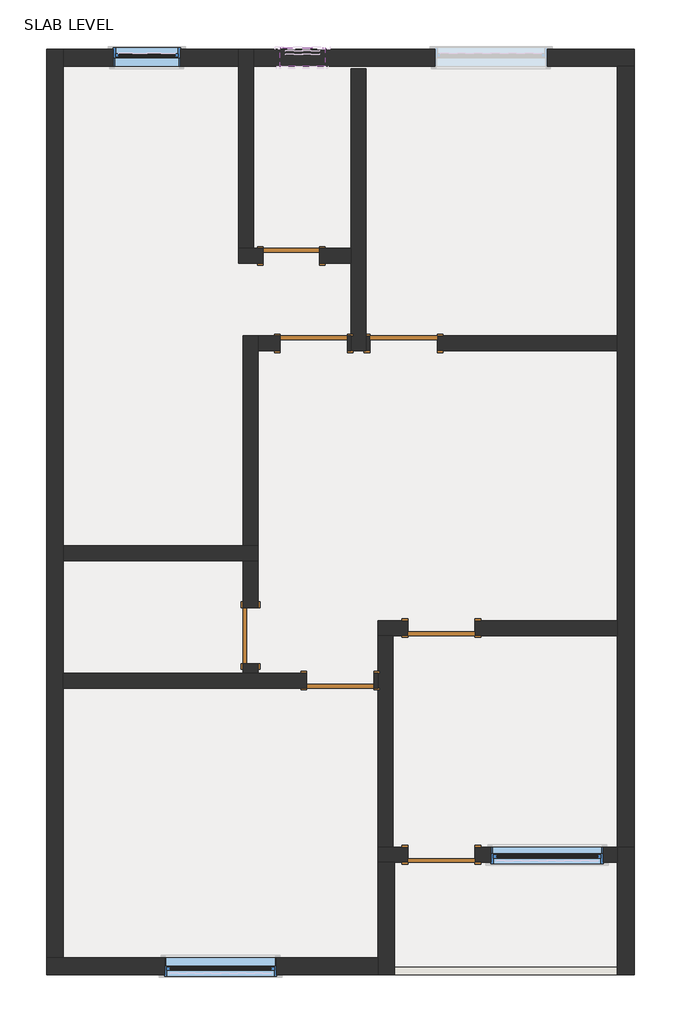
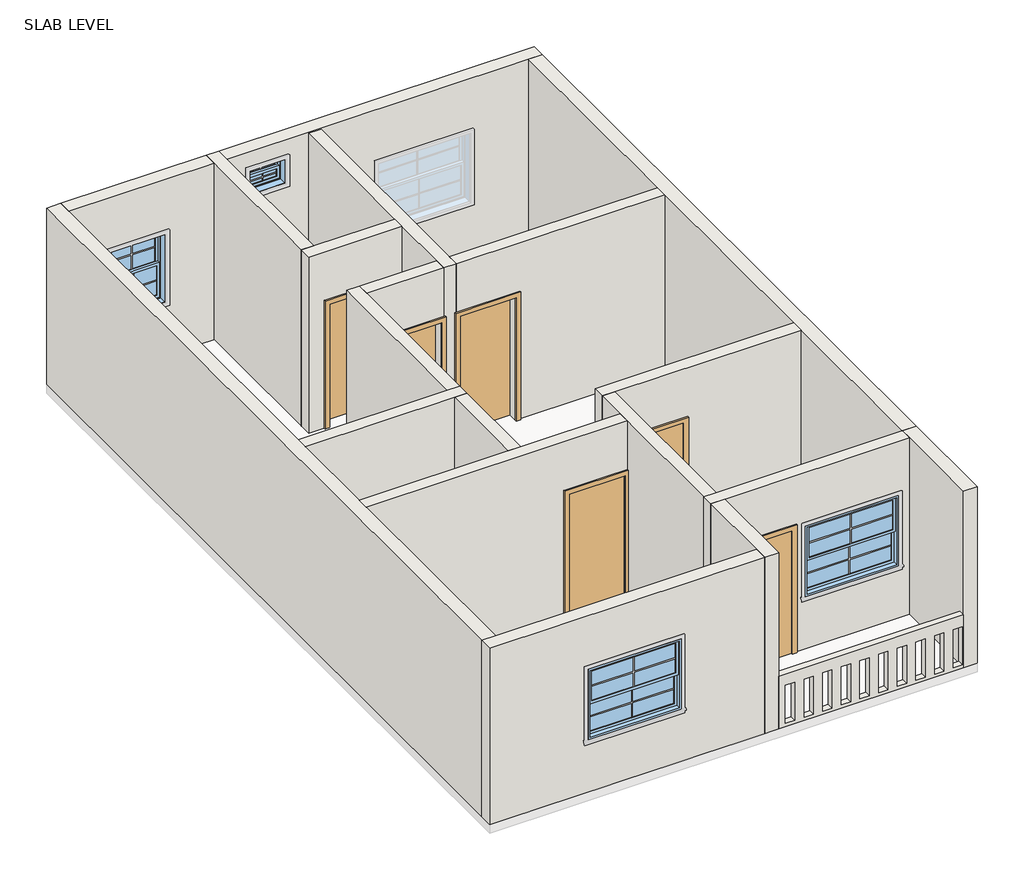
# One storey, part 1 of 2: 20 walls, 7 doors, 4 windows.
"""IFC4 building model written with IfcOpenShell, lengths in millimetres."""

from ifc_helpers import new_model, si_unit, frame, origin, place, context, project, spatial, polyline, outline, extrude, faceted_brep, transform, mapped, element, save
from components import door_4314e8ec, door_719f80de, door_54dd4da4, window_42222e0e, window_559c395e, window_a144fa31, window_d7d477dd

model = new_model("IFC4")

# Units and contexts
model_context = context("Model", 3, world=origin())
ifc_project = project(units=[si_unit("LENGTHUNIT", "METRE", prefix="MILLI")], contexts=[model_context])

# Site, building, storey
site = spatial("IfcSite", under=ifc_project)
building = spatial("IfcBuilding", under=site)
storey = spatial("IfcBuildingStorey", under=building, Name="SLAB LEVEL", Elevation=3048.0)

# Doors
placement = place(None, origin())
door_shape = door_4314e8ec(model_context)
element("IfcDoor", 1, ObjectType="Single-Flush : 30\" x 84\"", at=placement, inside=storey, context=model_context, shape_type="MappedRepresentation", body=[
    mapped(door_shape, transform((-5161.1019453, 13719.2944012, 3048.0), x_axis=(-1.0, 0.0, 0.0), y_axis=(0.0, -1.0, 0.0), z_axis=(0.0, 0.0, 1.0))),
])
element("IfcDoor", 2, ObjectType="Single-Flush : 30\" x 84\"", at=placement, inside=storey, context=model_context, shape_type="MappedRepresentation", body=[
    mapped(door_shape, transform((-5713.5519453, 8569.4444012, 3048.0), x_axis=(0.0, -1.0, 0.0), y_axis=(1.0, 0.0, 0.0), z_axis=(0.0, 0.0, 1.0))),
])
door_2_shape = door_719f80de(model_context)
element("IfcDoor", 3, ObjectType="Single-Flush : 36\" x 84\"", at=placement, inside=storey, context=model_context, shape_type="MappedRepresentation", body=[
    mapped(door_2_shape, transform((-3637.1019453, 12531.8444012, 3048.0), x_axis=(-1.0, 0.0, 0.0), y_axis=(0.0, -1.0, 0.0), z_axis=(0.0, 0.0, 1.0))),
])
door_3_shape = door_54dd4da4(model_context)
element("IfcDoor", 4, ObjectType="Single-Flush : 36\" x 84\"", at=placement, inside=storey, context=model_context, shape_type="MappedRepresentation", body=[
    mapped(door_3_shape, transform((-3122.7519453, 5597.6444012, 3048.0), x_axis=(-1.0, 0.0, 0.0), y_axis=(0.0, -1.0, 0.0), z_axis=(0.0, 0.0, 1.0))),
])
element("IfcDoor", 5, ObjectType="Single-Flush : 36\" x 84\"", at=placement, inside=storey, context=model_context, shape_type="MappedRepresentation", body=[
    mapped(door_3_shape, transform((-4494.3519453, 7959.8444012, 3048.0), x_axis=(-1.0, 0.0, 0.0), y_axis=(0.0, -1.0, 0.0), z_axis=(0.0, 0.0, 1.0))),
])
element("IfcDoor", 6, ObjectType="Single-Flush : 36\" x 84\"", at=placement, inside=storey, context=model_context, shape_type="MappedRepresentation", body=[
    mapped(door_3_shape, transform((-4856.3019453, 12531.8444012, 3048.0), x_axis=(1.0, 0.0, 0.0), y_axis=(0.0, 1.0, 0.0), z_axis=(0.0, 0.0, 1.0))),
])
element("IfcDoor", 7, ObjectType="Single-Flush : 36\" x 84\"", at=placement, inside=storey, context=model_context, shape_type="MappedRepresentation", body=[
    mapped(door_3_shape, transform((-3122.7519453, 8671.0444012, 3048.0), x_axis=(-1.0, 0.0, 0.0), y_axis=(0.0, -1.0, 0.0), z_axis=(0.0, 0.0, 1.0))),
])

# Walls
element("IfcWall", 8, ObjectType="WALL 4\"", at=placement, inside=storey, context=model_context, shape_type="SweptSolid", body=[
    extrude(outline(polyline([(3048.0, -3757.7519453), (3048.0, -735.1519453), (3962.4, -735.1519453), (3962.4, -3757.7519453), (3048.0, -3757.7519453)]), holes=[polyline([(3763.5002579, -3646.8161034), (3763.5002579, -3494.4161034), (3103.1002579, -3494.4161034), (3103.1002579, -3646.8161034), (3763.5002579, -3646.8161034)]), polyline([(3763.5002579, -3342.0161034), (3763.5002579, -3189.6161034), (3103.1002579, -3189.6161034), (3103.1002579, -3342.0161034), (3763.5002579, -3342.0161034)]), polyline([(3763.5002579, -3037.2161034), (3763.5002579, -2884.8161034), (3103.1002579, -2884.8161034), (3103.1002579, -3037.2161034), (3763.5002579, -3037.2161034)]), polyline([(3763.5002579, -2732.4161034), (3763.5002579, -2580.0161034), (3103.1002579, -2580.0161034), (3103.1002579, -2732.4161034), (3763.5002579, -2732.4161034)]), polyline([(3763.5002579, -2427.6161034), (3763.5002579, -2275.2161034), (3103.1002579, -2275.2161034), (3103.1002579, -2427.6161034), (3763.5002579, -2427.6161034)]), polyline([(3763.5002579, -2122.8161034), (3763.5002579, -1970.4161034), (3103.1002579, -1970.4161034), (3103.1002579, -2122.8161034), (3763.5002579, -2122.8161034)]), polyline([(3763.5002579, -1818.0161034), (3763.5002579, -1665.6161034), (3103.1002579, -1665.6161034), (3103.1002579, -1818.0161034), (3763.5002579, -1818.0161034)]), polyline([(3763.5002579, -1513.2161034), (3763.5002579, -1360.8161034), (3103.1002579, -1360.8161034), (3103.1002579, -1513.2161034), (3763.5002579, -1513.2161034)]), polyline([(3763.5002579, -1208.4161034), (3763.5002579, -1056.0161034), (3103.1002579, -1056.0161034), (3103.1002579, -1208.4161034), (3763.5002579, -1208.4161034)]), polyline([(3763.5002579, -903.6161034), (3763.5002579, -751.2161034), (3103.1002579, -751.2161034), (3103.1002579, -903.6161034), (3763.5002579, -903.6161034)])]), frame((0.0, 3972.0444012, 0.0), z_axis=(0.0, 1.0, 0.0), x_axis=(0.0, 0.0, 1.0)), (0.0, 0.0, 1.0), 101.6),
])
element("IfcWall", 9, ObjectType="WALL 6\"", at=placement, inside=storey, context=model_context, shape_type="Brep", body=[
    faceted_brep([(-4348.3019453, 16259.2944012, 3048.0), (-4348.3019453, 13820.8944012, 3048.0), (-4348.3019453, 13617.6944012, 3048.0), (-4348.3019453, 12633.4444012, 3048.0), (-4348.3019453, 12430.2444012, 3048.0), (-4348.3019453, 12430.2444012, 6096.0), (-4348.3019453, 12633.4444012, 6096.0), (-4348.3019453, 13617.6944012, 6096.0), (-4348.3019453, 13820.8944012, 6096.0), (-4348.3019453, 16259.2944012, 6096.0), (-4145.1019453, 16259.2944012, 3048.0), (-4145.1019453, 16259.2944012, 6096.0), (-4145.1019453, 12633.4444012, 6096.0), (-4145.1019453, 12430.2444012, 6096.0), (-4145.1019453, 12430.2444012, 3048.0), (-4145.1019453, 12633.4444012, 3048.0)], [[[0, 1, 2, 3, 4, 5, 6, 7, 8, 9]], [[10, 11, 12, 13, 14, 15]], [[4, 3, 2, 1, 0, 10, 15, 14]], [[9, 8, 7, 6, 5, 13, 12, 11]], [[0, 9, 11, 10]], [[5, 4, 14, 13]]]),
])
element("IfcWall", 10, ObjectType="WALL 6\"", at=placement, inside=storey, context=model_context, shape_type="Brep", body=[
    faceted_brep([(-5542.1019453, 13820.8944012, 5181.6), (-5542.1019453, 13820.8944012, 3048.0), (-5669.1019453, 13820.8944012, 3048.0), (-5872.3019453, 13820.8944012, 3048.0), (-5872.3019453, 13820.8944012, 6096.0), (-5669.1019453, 13820.8944012, 6096.0), (-4348.3019453, 13820.8944012, 6096.0), (-4348.3019453, 13820.8944012, 3048.0), (-4780.1019453, 13820.8944012, 3048.0), (-4780.1019453, 13820.8944012, 5181.6), (-5872.3019453, 13617.6944012, 3048.0), (-5542.1019453, 13617.6944012, 3048.0), (-5542.1019453, 13617.6944012, 5181.6), (-4780.1019453, 13617.6944012, 5181.6), (-4780.1019453, 13617.6944012, 3048.0), (-4348.3019453, 13617.6944012, 3048.0), (-4348.3019453, 13617.6944012, 6096.0), (-5872.3019453, 13617.6944012, 6096.0)], [[[0, 1, 2, 3, 4, 5, 6, 7, 8, 9]], [[10, 11, 12, 13, 14, 15, 16, 17]], [[8, 7, 15, 14]], [[3, 2, 1, 11, 10]], [[6, 5, 4, 17, 16]], [[4, 3, 10, 17]], [[7, 6, 16, 15]], [[12, 11, 1, 0]], [[13, 12, 0, 9]], [[14, 13, 9, 8]]]),
])
element("IfcWall", 11, ObjectType="WALL 6\"", at=placement, inside=storey, context=model_context, shape_type="Brep", body=[
    faceted_brep([(-5669.1019453, 13820.8944012, 3048.0), (-5669.1019453, 16291.0444012, 3048.0), (-5669.1019453, 16519.6444012, 3048.0), (-5669.1019453, 16519.6444012, 6096.0), (-5669.1019453, 16291.0444012, 6096.0), (-5669.1019453, 13820.8944012, 6096.0), (-5872.3019453, 13820.8944012, 3048.0), (-5872.3019453, 13820.8944012, 6096.0), (-5872.3019453, 16291.0444012, 6096.0), (-5872.3019453, 16519.6444012, 6096.0), (-5872.3019453, 16519.6444012, 3048.0), (-5872.3019453, 16291.0444012, 3048.0)], [[[0, 1, 2, 3, 4, 5]], [[6, 7, 8, 9, 10, 11]], [[2, 1, 0, 6, 11, 10]], [[5, 4, 3, 9, 8, 7]], [[0, 5, 7, 6]], [[3, 2, 10, 9]]]),
])
element("IfcWall", 12, ObjectType="WALL 6\"", at=placement, inside=storey, context=model_context, shape_type="SweptSolid", body=[
    extrude(outline(polyline([(3048.0, -4145.1019453), (3048.0, -4094.3019453), (5181.6, -4094.3019453), (5181.6, -3179.9019453), (3048.0, -3179.9019453), (3048.0, -735.1519453), (6096.0, -735.1519453), (6096.0, -4145.1019453), (3048.0, -4145.1019453)])), frame((0.0, 12430.2444012, 0.0), z_axis=(0.0, 1.0, 0.0), x_axis=(0.0, 0.0, 1.0)), (0.0, 0.0, 1.0), 203.2),
])
element("IfcWall", 13, ObjectType="WALL 6\"", at=placement, inside=storey, context=model_context, shape_type="Brep", body=[
    faceted_brep([(-3579.9519453, 8772.6444012, 5181.6), (-3579.9519453, 8772.6444012, 3048.0), (-3986.3519453, 8772.6444012, 3048.0), (-3986.3519453, 8772.6444012, 6096.0), (-735.1519453, 8772.6444012, 6096.0), (-735.1519453, 8772.6444012, 3048.0), (-2665.5519453, 8772.6444012, 3048.0), (-2665.5519453, 8772.6444012, 5181.6), (-3986.3519453, 8569.4444012, 3048.0), (-3783.1519453, 8569.4444012, 3048.0), (-3579.9519453, 8569.4444012, 3048.0), (-3579.9519453, 8569.4444012, 5181.6), (-2665.5519453, 8569.4444012, 5181.6), (-2665.5519453, 8569.4444012, 3048.0), (-735.1519453, 8569.4444012, 3048.0), (-735.1519453, 8569.4444012, 6096.0), (-3783.1519453, 8569.4444012, 6096.0), (-3986.3519453, 8569.4444012, 6096.0)], [[[0, 1, 2, 3, 4, 5, 6, 7]], [[8, 9, 10, 11, 12, 13, 14, 15, 16, 17]], [[6, 5, 14, 13]], [[2, 1, 10, 9, 8]], [[4, 3, 17, 16, 15]], [[5, 4, 15, 14]], [[3, 2, 8, 17]], [[11, 10, 1, 0]], [[12, 11, 0, 7]], [[13, 12, 7, 6]]]),
])
element("IfcWall", 14, ObjectType="WALL 6\"", at=placement, inside=storey, context=model_context, shape_type="Brep", body=[
    faceted_brep([(-3579.9519453, 5699.2444012, 5181.6), (-3579.9519453, 5699.2444012, 3048.0), (-3783.1519453, 5699.2444012, 3048.0), (-3986.3519453, 5699.2444012, 3048.0), (-3986.3519453, 5699.2444012, 6096.0), (-3783.1519453, 5699.2444012, 6096.0), (-735.1519453, 5699.2444012, 6096.0), (-735.1519453, 5699.2444012, 3048.0), (-2665.5519453, 5699.2444012, 3048.0), (-2665.5519453, 5699.2444012, 5181.6), (-925.6519453, 5699.2444012, 5181.6), (-2449.6519453, 5699.2444012, 5181.6), (-2449.6519453, 5699.2444012, 3962.4), (-925.6519453, 5699.2444012, 3962.4), (-3986.3519453, 5496.0444012, 3048.0), (-3757.7519453, 5496.0444012, 3048.0), (-3579.9519453, 5496.0444012, 3048.0), (-3579.9519453, 5496.0444012, 5181.6), (-2665.5519453, 5496.0444012, 5181.6), (-2665.5519453, 5496.0444012, 3048.0), (-735.1519453, 5496.0444012, 3048.0), (-735.1519453, 5496.0444012, 6096.0), (-3757.7519453, 5496.0444012, 6096.0), (-3986.3519453, 5496.0444012, 6096.0), (-925.6519453, 5496.0444012, 5181.6), (-925.6519453, 5496.0444012, 3962.4), (-2449.6519453, 5496.0444012, 3962.4), (-2449.6519453, 5496.0444012, 5181.6)], [[[0, 1, 2, 3, 4, 5, 6, 7, 8, 9], [10, 11, 12, 13]], [[14, 15, 16, 17, 18, 19, 20, 21, 22, 23], [24, 25, 26, 27]], [[8, 7, 20, 19]], [[3, 2, 1, 16, 15, 14]], [[6, 5, 4, 23, 22, 21]], [[7, 6, 21, 20]], [[4, 3, 14, 23]], [[17, 16, 1, 0]], [[18, 17, 0, 9]], [[19, 18, 9, 8]], [[25, 24, 10, 13]], [[26, 25, 13, 12]], [[27, 26, 12, 11]], [[24, 27, 11, 10]]]),
])
element("IfcWall", 15, ObjectType="WALL 6\"", at=placement, inside=storey, context=model_context, shape_type="Brep", body=[
    faceted_brep([(-3783.1519453, 5699.2444012, 3048.0), (-3783.1519453, 8569.4444012, 3048.0), (-3783.1519453, 8569.4444012, 6096.0), (-3783.1519453, 5699.2444012, 6096.0), (-3986.3519453, 5699.2444012, 3048.0), (-3986.3519453, 5699.2444012, 6096.0), (-3986.3519453, 7858.2444012, 6096.0), (-3986.3519453, 8061.4444012, 6096.0), (-3986.3519453, 8569.4444012, 6096.0), (-3986.3519453, 8569.4444012, 3048.0), (-3986.3519453, 8061.4444012, 3048.0), (-3986.3519453, 7858.2444012, 3048.0)], [[[0, 1, 2, 3]], [[4, 5, 6, 7, 8, 9, 10, 11]], [[1, 0, 4, 11, 10, 9]], [[3, 2, 8, 7, 6, 5]], [[0, 3, 5, 4]], [[2, 1, 9, 8]]]),
])
element("IfcWall", 16, ObjectType="WALL 6\"", at=placement, inside=storey, context=model_context, shape_type="Brep", body=[
    faceted_brep([(-8253.5519453, 7858.2444012, 3048.0), (-4951.5519453, 7858.2444012, 3048.0), (-4951.5519453, 7858.2444012, 5181.6), (-4037.1519453, 7858.2444012, 5181.6), (-4037.1519453, 7858.2444012, 3048.0), (-3986.3519453, 7858.2444012, 3048.0), (-3986.3519453, 7858.2444012, 6096.0), (-8253.5519453, 7858.2444012, 6096.0), (-4951.5519453, 8061.4444012, 5181.6), (-4951.5519453, 8061.4444012, 3048.0), (-5611.9519453, 8061.4444012, 3048.0), (-5815.1519453, 8061.4444012, 3048.0), (-8253.5519453, 8061.4444012, 3048.0), (-8253.5519453, 8061.4444012, 6096.0), (-5815.1519453, 8061.4444012, 6096.0), (-5611.9519453, 8061.4444012, 6096.0), (-3986.3519453, 8061.4444012, 6096.0), (-3986.3519453, 8061.4444012, 3048.0), (-4037.1519453, 8061.4444012, 3048.0), (-4037.1519453, 8061.4444012, 5181.6)], [[[0, 1, 2, 3, 4, 5, 6, 7]], [[8, 9, 10, 11, 12, 13, 14, 15, 16, 17, 18, 19]], [[18, 17, 5, 4]], [[12, 11, 10, 9, 1, 0]], [[7, 6, 16, 15, 14, 13]], [[0, 7, 13, 12]], [[6, 5, 17, 16]], [[2, 1, 9, 8]], [[3, 2, 8, 19]], [[4, 3, 19, 18]]]),
])
element("IfcWall", 17, ObjectType="WALL 6\"", at=placement, inside=storey, context=model_context, shape_type="Brep", body=[
    faceted_brep([(-8253.5519453, 9585.4444012, 3048.0), (-5815.1519453, 9585.4444012, 3048.0), (-5611.9519453, 9585.4444012, 3048.0), (-5611.9519453, 9585.4444012, 6096.0), (-5815.1519453, 9585.4444012, 6096.0), (-8253.5519453, 9585.4444012, 6096.0), (-8253.5519453, 9788.6444012, 3048.0), (-8253.5519453, 9788.6444012, 6096.0), (-5815.1519453, 9788.6444012, 6096.0), (-5611.9519453, 9788.6444012, 6096.0), (-5611.9519453, 9788.6444012, 3048.0), (-5815.1519453, 9788.6444012, 3048.0)], [[[0, 1, 2, 3, 4, 5]], [[6, 7, 8, 9, 10, 11]], [[2, 1, 0, 6, 11, 10]], [[5, 4, 3, 9, 8, 7]], [[0, 5, 7, 6]], [[3, 2, 10, 9]]]),
])
element("IfcWall", 18, ObjectType="WALL 6\"", at=placement, inside=storey, context=model_context, shape_type="SweptSolid", body=[
    extrude(outline(polyline([(8188.4444012, 5181.6), (8188.4444012, 3048.0), (8061.4444012, 3048.0), (8061.4444012, 6096.0), (9585.4444012, 6096.0), (9585.4444012, 3048.0), (8950.4444012, 3048.0), (8950.4444012, 5181.6), (8188.4444012, 5181.6)])), frame((-5815.1519453, 0.0, 0.0), z_axis=(1.0, 0.0, 0.0), x_axis=(0.0, 1.0, 0.0)), (0.0, 0.0, 1.0), 203.2),
])
element("IfcWall", 19, ObjectType="WALL 6\"", at=placement, inside=storey, context=model_context, shape_type="Brep", body=[
    faceted_brep([(-5611.9519453, 9788.6444012, 3048.0), (-5611.9519453, 12430.2444012, 3048.0), (-5611.9519453, 12633.4444012, 3048.0), (-5611.9519453, 12633.4444012, 6096.0), (-5611.9519453, 12430.2444012, 6096.0), (-5611.9519453, 9788.6444012, 6096.0), (-5815.1519453, 9788.6444012, 3048.0), (-5815.1519453, 9788.6444012, 6096.0), (-5815.1519453, 12633.4444012, 6096.0), (-5815.1519453, 12633.4444012, 3048.0)], [[[0, 1, 2, 3, 4, 5]], [[6, 7, 8, 9]], [[2, 1, 0, 6, 9]], [[5, 4, 3, 8, 7]], [[0, 5, 7, 6]], [[3, 2, 9, 8]]]),
])
element("IfcWall", 20, ObjectType="WALL 6\"", at=placement, inside=storey, context=model_context, shape_type="SweptSolid", body=[
    extrude(outline(polyline([(5181.6, -4399.1019453), (3048.0, -4399.1019453), (3048.0, -4348.3019453), (6096.0, -4348.3019453), (6096.0, -5611.9519453), (3048.0, -5611.9519453), (3048.0, -5313.5019453), (5181.6, -5313.5019453), (5181.6, -4399.1019453)])), frame((0.0, 12430.2444012, 0.0), z_axis=(0.0, 1.0, 0.0), x_axis=(0.0, 0.0, 1.0)), (0.0, 0.0, 1.0), 203.2),
])
element("IfcWall", 21, ObjectType="WALL 9\"", at=placement, inside=storey, context=model_context, shape_type="Brep", body=[
    faceted_brep([(-506.5519453, 16519.6444012, 6096.0), (-506.5519453, 16519.6444012, 3048.0), (-5669.1019453, 16519.6444012, 3048.0), (-5669.1019453, 16519.6444012, 6096.0), (-3211.6519453, 16519.6444012, 5181.6), (-3211.6519453, 16519.6444012, 3962.4), (-1687.6519453, 16519.6444012, 3962.4), (-1687.6519453, 16519.6444012, 5181.6), (-5313.5019453, 16519.6444012, 5791.2), (-5313.5019453, 16519.6444012, 5334.0), (-4703.9019453, 16519.6444012, 5334.0), (-4703.9019453, 16519.6444012, 5791.2), (-506.5519453, 16291.0444012, 3048.0), (-506.5519453, 16291.0444012, 6096.0), (-735.1519453, 16291.0444012, 6096.0), (-5669.1019453, 16291.0444012, 6096.0), (-5669.1019453, 16291.0444012, 3048.0), (-735.1519453, 16291.0444012, 3048.0), (-3211.6519453, 16291.0444012, 5181.6), (-1687.6519453, 16291.0444012, 5181.6), (-1687.6519453, 16291.0444012, 3962.4), (-3211.6519453, 16291.0444012, 3962.4), (-5313.5019453, 16291.0444012, 5791.2), (-4703.9019453, 16291.0444012, 5791.2), (-4703.9019453, 16291.0444012, 5334.0), (-5313.5019453, 16291.0444012, 5334.0)], [[[0, 1, 2, 3], [4, 5, 6, 7], [8, 9, 10, 11]], [[12, 13, 14, 15, 16, 17], [18, 19, 20, 21], [22, 23, 24, 25]], [[2, 1, 12, 17, 16]], [[0, 3, 15, 14, 13]], [[3, 2, 16, 15]], [[5, 4, 18, 21]], [[6, 5, 21, 20]], [[7, 6, 20, 19]], [[4, 7, 19, 18]], [[9, 8, 22, 25]], [[10, 9, 25, 24]], [[11, 10, 24, 23]], [[8, 11, 23, 22]], [[0, 13, 12, 1]]]),
])
element("IfcWall", 22, ObjectType="WALL 9\"", at=placement, inside=storey, context=model_context, shape_type="Brep", body=[
    faceted_brep([(-735.1519453, 16291.0444012, 6096.0), (-735.1519453, 16291.0444012, 3048.0), (-735.1519453, 12633.4444012, 3048.0), (-735.1519453, 12430.2444012, 3048.0), (-735.1519453, 8772.6444012, 3048.0), (-735.1519453, 8569.4444012, 3048.0), (-735.1519453, 5699.2444012, 3048.0), (-735.1519453, 5699.2444012, 6096.0), (-735.1519453, 8569.4444012, 6096.0), (-735.1519453, 8772.6444012, 6096.0), (-735.1519453, 12430.2444012, 6096.0), (-735.1519453, 12633.4444012, 6096.0), (-506.5519453, 16291.0444012, 3048.0), (-506.5519453, 16291.0444012, 6096.0), (-506.5519453, 5699.2444012, 6096.0), (-506.5519453, 5699.2444012, 3048.0)], [[[0, 1, 2, 3, 4, 5, 6, 7, 8, 9, 10, 11]], [[12, 13, 14, 15]], [[6, 5, 4, 3, 2, 1, 12, 15]], [[0, 11, 10, 9, 8, 7, 14, 13]], [[7, 6, 15, 14]], [[0, 13, 12, 1]]]),
])
element("IfcWall", 23, ObjectType="WALL 9\"", at=placement, inside=storey, context=model_context, shape_type="Brep", body=[
    faceted_brep([(-506.5519453, 3972.0444012, 3048.0), (-506.5519453, 5699.2444012, 3048.0), (-506.5519453, 5699.2444012, 6096.0), (-506.5519453, 3972.0444012, 6096.0), (-735.1519453, 3972.0444012, 3048.0), (-735.1519453, 3972.0444012, 3962.4), (-735.1519453, 3972.0444012, 6096.0), (-735.1519453, 5496.0444012, 6096.0), (-735.1519453, 5699.2444012, 6096.0), (-735.1519453, 5699.2444012, 3048.0), (-735.1519453, 5496.0444012, 3048.0), (-735.1519453, 4073.6444012, 3048.0)], [[[0, 1, 2, 3]], [[4, 5, 6, 7, 8, 9, 10, 11]], [[1, 0, 4, 11, 10, 9]], [[3, 2, 8, 7, 6]], [[2, 1, 9, 8]], [[0, 3, 6, 5, 4]]]),
])
element("IfcWall", 24, ObjectType="WALL 9\"", at=placement, inside=storey, context=model_context, shape_type="Brep", body=[
    faceted_brep([(-3986.3519453, 5496.0444012, 3048.0), (-3986.3519453, 4200.6444012, 3048.0), (-3986.3519453, 3972.0444012, 3048.0), (-3986.3519453, 3972.0444012, 6096.0), (-3986.3519453, 4200.6444012, 6096.0), (-3986.3519453, 5496.0444012, 6096.0), (-3757.7519453, 5496.0444012, 3048.0), (-3757.7519453, 5496.0444012, 6096.0), (-3757.7519453, 3972.0444012, 6096.0), (-3757.7519453, 3972.0444012, 3962.4), (-3757.7519453, 3972.0444012, 3048.0), (-3757.7519453, 4073.6444012, 3048.0)], [[[0, 1, 2, 3, 4, 5]], [[6, 7, 8, 9, 10, 11]], [[2, 1, 0, 6, 11, 10]], [[5, 4, 3, 8, 7]], [[0, 5, 7, 6]], [[2, 10, 9, 8, 3]]]),
])
element("IfcWall", 25, ObjectType="WALL 9\"", at=placement, inside=storey, context=model_context, shape_type="Brep", body=[
    faceted_brep([(-3986.3519453, 4200.6444012, 6096.0), (-3986.3519453, 4200.6444012, 3048.0), (-8253.5519453, 4200.6444012, 3048.0), (-8482.1519453, 4200.6444012, 3048.0), (-8482.1519453, 4200.6444012, 6096.0), (-8253.5519453, 4200.6444012, 6096.0), (-5357.9519453, 4200.6444012, 5181.6), (-6881.9519453, 4200.6444012, 5181.6), (-6881.9519453, 4200.6444012, 3962.4), (-5357.9519453, 4200.6444012, 3962.4), (-3986.3519453, 3972.0444012, 3048.0), (-3986.3519453, 3972.0444012, 6096.0), (-8482.1519453, 3972.0444012, 6096.0), (-8482.1519453, 3972.0444012, 3048.0), (-5357.9519453, 3972.0444012, 5181.6), (-5357.9519453, 3972.0444012, 3962.4), (-6881.9519453, 3972.0444012, 3962.4), (-6881.9519453, 3972.0444012, 5181.6)], [[[0, 1, 2, 3, 4, 5], [6, 7, 8, 9]], [[10, 11, 12, 13], [14, 15, 16, 17]], [[3, 2, 1, 10, 13]], [[0, 5, 4, 12, 11]], [[4, 3, 13, 12]], [[15, 14, 6, 9]], [[16, 15, 9, 8]], [[17, 16, 8, 7]], [[14, 17, 7, 6]], [[0, 11, 10, 1]]]),
])
element("IfcWall", 26, ObjectType="WALL 9\"", at=placement, inside=storey, context=model_context, shape_type="Brep", body=[
    faceted_brep([(-8253.5519453, 4200.6444012, 3048.0), (-8253.5519453, 7858.2444012, 3048.0), (-8253.5519453, 8061.4444012, 3048.0), (-8253.5519453, 9585.4444012, 3048.0), (-8253.5519453, 9788.6444012, 3048.0), (-8253.5519453, 16291.0444012, 3048.0), (-8253.5519453, 16519.6444012, 3048.0), (-8253.5519453, 16519.6444012, 3962.4), (-8253.5519453, 16519.6444012, 6096.0), (-8253.5519453, 16291.0444012, 6096.0), (-8253.5519453, 9788.6444012, 6096.0), (-8253.5519453, 9585.4444012, 6096.0), (-8253.5519453, 8061.4444012, 6096.0), (-8253.5519453, 7858.2444012, 6096.0), (-8253.5519453, 4200.6444012, 6096.0), (-8482.1519453, 4200.6444012, 3048.0), (-8482.1519453, 4200.6444012, 6096.0), (-8482.1519453, 16519.6444012, 6096.0), (-8482.1519453, 16519.6444012, 3048.0)], [[[0, 1, 2, 3, 4, 5, 6, 7, 8, 9, 10, 11, 12, 13, 14]], [[15, 16, 17, 18]], [[6, 5, 4, 3, 2, 1, 0, 15, 18]], [[14, 13, 12, 11, 10, 9, 8, 17, 16]], [[0, 14, 16, 15]], [[6, 18, 17, 8, 7]]]),
])
element("IfcWall", 27, ObjectType="WALL 9\"", at=placement, inside=storey, context=model_context, shape_type="SweptSolid", body=[
    extrude(outline(polyline([(6096.0, -8253.5519453), (3048.0, -8253.5519453), (3048.0, -5872.3019453), (6096.0, -5872.3019453), (6096.0, -8253.5519453)]), holes=[polyline([(5181.6, -7577.2769453), (5181.6, -6662.8769453), (3962.4, -6662.8769453), (3962.4, -7577.2769453), (5181.6, -7577.2769453)])]), frame((0.0, 16291.0444012, 0.0), z_axis=(0.0, 1.0, 0.0), x_axis=(0.0, 0.0, 1.0)), (0.0, 0.0, 1.0), 228.6),
])

# Windows
window_shape = window_42222e0e(model_context)
element("IfcWindow", 28, ObjectType="Window-Double-Hung : 24\" x 1'6\"", at=placement, inside=storey, context=model_context, shape_type="MappedRepresentation", body=[
    mapped(window_shape, transform((-5008.7019453, 16405.3444012, 4419.6), x_axis=(1.0, 0.0, 0.0), y_axis=(0.0, 1.0, 0.0), z_axis=(0.0, 0.0, 1.0))),
])
window_2_shape = window_559c395e(model_context)
element("IfcWindow", 29, ObjectType="Window-Double-Hung : 36\"X48\"", at=placement, inside=storey, context=model_context, shape_type="MappedRepresentation", body=[
    mapped(window_2_shape, transform((-7120.0769453, 16405.3444012, 3048.0), x_axis=(1.0, 0.0, 0.0), y_axis=(0.0, 1.0, 0.0), z_axis=(0.0, 0.0, 1.0))),
])
window_3_shape = window_a144fa31(model_context)
element("IfcWindow", 30, ObjectType="Window-Double-Hung : 60\"X48\"", at=placement, inside=storey, context=model_context, shape_type="MappedRepresentation", body=[
    mapped(window_3_shape, transform((-6119.9519453, 4086.3444012, 3048.0), x_axis=(-1.0, 0.0, 0.0), y_axis=(0.0, -1.0, 0.0), z_axis=(0.0, 0.0, 1.0))),
])
window_4_shape = window_d7d477dd(model_context)
element("IfcWindow", 31, ObjectType="Window-Double-Hung : 60\"X48\"", at=placement, inside=storey, context=model_context, shape_type="MappedRepresentation", body=[
    mapped(window_4_shape, transform((-1687.6519453, 5597.6444012, 3048.0), x_axis=(-1.0, 0.0, 0.0), y_axis=(0.0, -1.0, 0.0), z_axis=(0.0, 0.0, 1.0))),
])

save(model, "model.ifc")

# Revit data of these elements
# Type "Single-Flush : 30\" x 84\""
#   Type Mark = "4"
#   Construction Type Id = "MDOOR"
#   Assembly Code = "C1020"
#   Analytic Construction = "Metal"
#   Thickness = 0' - 2"
#   Heat Transfer Coefficient (U) = 0.651978 BTU/(h·ft²·°F)
#   Height = 7' - 0"
#   Trim Projection Ext = 0' - 1"
#   Trim Projection Int = 0' - 1"
#   Trim Width = 0' - 3"
#   Width = 2' - 6"
#   Define Thermal Properties by = 1
#   Define Thermal Properties by = 1
#   Door Material = Door - Panel
#   Frame Material = Door - Frame
#   Visual Light Transmittance = 0
#   Solar Heat Gain Coefficient = 0
#   Function = (empty or 0)
#   Wall Closure = (empty or 0)
# Type "Single-Flush : 36\" x 84\""
#   Type Mark = "1"
#   Construction Type Id = "MDOOR"
#   Assembly Code = "C1020"
#   Analytic Construction = "Metal"
#   Thickness = 0' - 2"
#   Heat Transfer Coefficient (U) = 0.651978 BTU/(h·ft²·°F)
#   Height = 7' - 0"
#   Trim Projection Ext = 0' - 1"
#   Trim Projection Int = 0' - 1"
#   Trim Width = 0' - 3"
#   Width = 3' - 0"
#   Define Thermal Properties by = 1
#   Define Thermal Properties by = 1
#   Door Material = Door - Panel
#   Frame Material = Door - Frame
#   Visual Light Transmittance = 0
#   Solar Heat Gain Coefficient = 0
#   Function = (empty or 0)
#   Wall Closure = (empty or 0)
# Type "WALL 4\""
#   Assembly Code = "B2010"
#   Layers, outside or top first: 0' - 4" no material (function 1)
# Type "WALL 6\""
#   Assembly Code = "B2010"
#   Layers, outside or top first: 0' - 8" no material (function 1)
# Type "WALL 9\""
#   Assembly Code = "B2010"
#   Layers, outside or top first: 0' - 9" no material (function 1)
# Type "Window-Double-Hung : 24\" x 1'6\""
#   Type Mark = "19"
#   Fire Rating = "0.5h"
#   Construction Type Id = "DG-DR"
#   Assembly Code = "B2020100"
#   Analytic Construction = "Double glazing - domestic"
#   Wall Thickness [instance default] = 0' - 6"
#   Window Inset [instance default] = 0' - 0"
#   Visual Light Transmittance = 0.81
#   Thermal Resistance (R) = 1.8146 (h·ft²·°F)/BTU
#   Solar Heat Gain Coefficient = 0.76
#   Muntin Width = 1' - 6"
#   Muntin Height = 0' - 5 1/8"
#   Interior Wall Closure [instance default] = 0' - 1 1/2"
#   Rough Width = 2' - 0 1/2"
#   Rough Height = 1' - 6 1/2"
#   Frame Extension [instance default] = 0' - 1 1/4"
#   Exterior Wall Closure [instance default] = 0' - 0 1/2"
#   Extension Jamb [instance default] = 0' - 1 1/2"
#   Heat Transfer Coefficient (U) = 0.5511 BTU/(h·ft²·°F)
#   Height = 1' - 6"
#   Width = 2' - 0"
#   Top Muntin Visibility = yes
#   Indicator Visibility [instance default] = yes
#   Extension Jamb Visibility [instance default] = yes
#   Interior Trim Visibility [instance default] = yes
#   Exterior Trim Visibility [instance default] = yes
#   Define Thermal Properties by = 1
#   Bottom Muntin Visibility = yes
#   Muntin Pattern = Muntin Pattern_2x2 : Muntin Pattern_2x2
#   Interior Trim Material = Wood - Stained
#   Interior Trim = Trim-Window-Interior-Flat : Picture Frame
#   Exterior Trim Material = Clad - White
#   Exterior Trim = Trim-Window-Exterior-Flat : with Sill
#   Glass Panel Material = Glass
#   Exterior Frame Material = Clad - White
#   Interior Frame Material = Wood - Stained
#   Wall Closure = (empty or 0)
# Type "Window-Double-Hung : 36\"X48\""
#   Type Mark = "21"
#   Fire Rating = "0.5h"
#   Construction Type Id = "DG-DR"
#   Assembly Code = "B2020100"
#   Analytic Construction = "Double glazing - domestic"
#   Wall Thickness [instance default] = 0' - 6"
#   Window Inset [instance default] = 0' - 0"
#   Visual Light Transmittance = 0.81
#   Thermal Resistance (R) = 1.8146 (h·ft²·°F)/BTU
#   Solar Heat Gain Coefficient = 0.76
#   Muntin Width = 2' - 6"
#   Muntin Height = 1' - 8 1/8"
#   Interior Wall Closure [instance default] = 0' - 1 1/2"
#   Rough Width = 3' - 0 1/2"
#   Rough Height = 4' - 0 1/2"
#   Frame Extension [instance default] = 0' - 1 1/4"
#   Exterior Wall Closure [instance default] = 0' - 0 1/2"
#   Extension Jamb [instance default] = 0' - 1 1/2"
#   Heat Transfer Coefficient (U) = 0.5511 BTU/(h·ft²·°F)
#   Height = 4' - 0"
#   Width = 3' - 0"
#   Top Muntin Visibility = yes
#   Indicator Visibility [instance default] = yes
#   Extension Jamb Visibility [instance default] = yes
#   Interior Trim Visibility [instance default] = yes
#   Exterior Trim Visibility [instance default] = yes
#   Define Thermal Properties by = 1
#   Bottom Muntin Visibility = yes
#   Muntin Pattern = Muntin Pattern_2x2 : Muntin Pattern_2x2
#   Interior Trim Material = Wood - Stained
#   Interior Trim = Trim-Window-Interior-Flat : Picture Frame
#   Exterior Trim Material = Clad - White
#   Exterior Trim = Trim-Window-Exterior-Flat : with Sill
#   Glass Panel Material = Glass
#   Exterior Frame Material = Clad - White
#   Interior Frame Material = Wood - Stained
#   Wall Closure = (empty or 0)
# Type "Window-Double-Hung : 60\"X48\""
#   Type Mark = "18"
#   Fire Rating = "0.5h"
#   Construction Type Id = "DG-DR"
#   Assembly Code = "B2020100"
#   Analytic Construction = "Double glazing - domestic"
#   Wall Thickness [instance default] = 0' - 6"
#   Window Inset [instance default] = 0' - 0"
#   Visual Light Transmittance = 0.81
#   Thermal Resistance (R) = 1.8146 (h·ft²·°F)/BTU
#   Solar Heat Gain Coefficient = 0.76
#   Muntin Width = 4' - 6"
#   Muntin Height = 1' - 8 1/8"
#   Interior Wall Closure [instance default] = 0' - 1 1/2"
#   Rough Width = 5' - 0 1/2"
#   Rough Height = 4' - 0 1/2"
#   Frame Extension [instance default] = 0' - 1 1/4"
#   Exterior Wall Closure [instance default] = 0' - 0 1/2"
#   Extension Jamb [instance default] = 0' - 1 1/2"
#   Heat Transfer Coefficient (U) = 0.5511 BTU/(h·ft²·°F)
#   Height = 4' - 0"
#   Width = 5' - 0"
#   Top Muntin Visibility = yes
#   Indicator Visibility [instance default] = yes
#   Extension Jamb Visibility [instance default] = yes
#   Interior Trim Visibility [instance default] = yes
#   Exterior Trim Visibility [instance default] = yes
#   Define Thermal Properties by = 1
#   Bottom Muntin Visibility = yes
#   Muntin Pattern = Muntin Pattern_2x2 : Muntin Pattern_2x2
#   Interior Trim Material = Wood - Stained
#   Interior Trim = Trim-Window-Interior-Flat : Picture Frame
#   Exterior Trim Material = Clad - White
#   Exterior Trim = Trim-Window-Exterior-Flat : with Sill
#   Glass Panel Material = Glass
#   Exterior Frame Material = Clad - White
#   Interior Frame Material = Wood - Stained
#   Wall Closure = (empty or 0)
# Elements 1, 2 (IfcDoor, "Single-Flush : 30\" x 84\"")
#   Phase Created = New Construction
#   Materials on its faces: "Door - Frame", "Door - Panel"
# Elements 3, 4, 5, 6, 7 (IfcDoor, "Single-Flush : 36\" x 84\"")
#   Phase Created = New Construction
#   Materials on its faces: "Door - Frame", "Door - Panel"
# Element 8 (IfcWall, "WALL 4\"")
#   Top Offset = 0' - 0"
#   Base Offset = 0' - 0"
#   wall height = 3' - 0"
#   Phase Created = New Construction
#   Base Constraint = SLAB LEVEL
#   Materials on its faces: "Default Wall"
# Elements 9, 10, 12, 13, 15, 16, 17, 18, 19, 20 (IfcWall, "WALL 6\"")
#   Top Offset = 0' - 0"
#   Base Offset = 0' - 0"
#   wall height = 10' - 0"
#   Phase Created = New Construction
#   Base Constraint = SLAB LEVEL
#   Top Constraint = FIRST FLOOR
#   Materials on its faces: "Default Wall"
# Element 11 (IfcWall, "WALL 6\"")
#   Top Offset = 0' - 0"
#   Base Offset = 0' - 0"
#   wall height = 10' - 0"
#   Phase Created = New Construction
#   Base Constraint = SLAB LEVEL
#   Top Constraint = FIRST FLOOR
#   Materials on its faces: "Default Wall", "1 wall paint"
# Element 14 (IfcWall, "WALL 6\"")
#   Top Offset = 0' - 0"
#   Base Offset = 0' - 0"
#   wall height = 10' - 0"
#   Phase Created = New Construction
#   Base Constraint = SLAB LEVEL
#   Top Constraint = FIRST FLOOR
#   Materials on its faces: "Default Wall", "Wood Planks"
# Elements 21, 22, 23, 26, 27 (IfcWall, "WALL 9\"")
#   Top Offset = 0' - 0"
#   Base Offset = 0' - 0"
#   wall height = 10' - 0"
#   Phase Created = New Construction
#   Base Constraint = SLAB LEVEL
#   Top Constraint = FIRST FLOOR
#   Materials on its faces: "Default Wall", "1 wall paint"
# Element 24 (IfcWall, "WALL 9\"")
#   Top Offset = 0' - 0"
#   Base Offset = 0' - 0"
#   wall height = 10' - 0"
#   Phase Created = New Construction
#   Base Constraint = SLAB LEVEL
#   Top Constraint = FIRST FLOOR
#   Materials on its faces: "Default Wall", "Wood Planks"
# Element 25 (IfcWall, "WALL 9\"")
#   Top Offset = 0' - 0"
#   Base Offset = 0' - 0"
#   wall height = 10' - 0"
#   Phase Created = New Construction
#   Base Constraint = SLAB LEVEL
#   Top Constraint = FIRST FLOOR
#   Materials on its faces: "Default Wall", "Wood Planks", "1 wall paint"
# Element 28 (IfcWindow, "Window-Double-Hung : 24\" x 1'6\"")
#   Mark = "10"
#   Window Inset = 0' - 0"
#   Interior Wall Closure = 0' - 1 1/2"
#   Frame Extension = 0' - 1 1/4"
#   Exterior Wall Closure = 0' - 0 1/2"
#   Interior Trim Visibility = yes
#   Indicator Visibility = yes
#   Exterior Trim Visibility = yes
#   Phase Created = New Construction
#   Materials on its faces: "Wood - Stained", "Glass", "Clad - White"
# Element 29 (IfcWindow, "Window-Double-Hung : 36\"X48\"")
#   Mark = "11"
#   Window Inset = 0' - 0"
#   Interior Wall Closure = 0' - 1 1/2"
#   Frame Extension = 0' - 1 1/4"
#   Exterior Wall Closure = 0' - 0 1/2"
#   Interior Trim Visibility = yes
#   Indicator Visibility = yes
#   Exterior Trim Visibility = yes
#   Phase Created = New Construction
#   Materials on its faces: "Wood - Stained", "Glass", "Clad - White"
# Element 30 (IfcWindow, "Window-Double-Hung : 60\"X48\"")
#   Mark = "8"
#   Window Inset = 0' - 0"
#   Interior Wall Closure = 0' - 1 1/2"
#   Frame Extension = 0' - 1 1/4"
#   Exterior Wall Closure = 0' - 0 1/2"
#   Interior Trim Visibility = yes
#   Indicator Visibility = yes
#   Exterior Trim Visibility = yes
#   Phase Created = New Construction
#   Materials on its faces: "Wood - Stained", "Glass", "Clad - White"
# Element 31 (IfcWindow, "Window-Double-Hung : 60\"X48\"")
#   Mark = "7"
#   Window Inset = 0' - 0"
#   Interior Wall Closure = 0' - 1 1/2"
#   Frame Extension = 0' - 1 1/4"
#   Exterior Wall Closure = 0' - 0 1/2"
#   Interior Trim Visibility = yes
#   Indicator Visibility = yes
#   Exterior Trim Visibility = yes
#   Phase Created = New Construction
#   Materials on its faces: "Wood - Stained", "Glass", "Clad - White"
# Materials
#   "Door - Panel": class "Wood", colour RGB 210 159 95, transparency 0, Cost = 0
#   "Door - Frame": colour RGB 118 70 51, transparency 0, Cost = 0
#   "Wood - Stained": class "Wood", colour RGB 224 178 126, transparency 0, Cost = 0
#   "Clad - White": class "Wood", colour RGB 242 242 238, transparency 0, Cost = 0
#   "Glass": class "Glass", colour RGB 0 128 192, transparency 0.75, Description = "Soda Lime Glass", Cost = 0
#   "Default Wall": colour RGB 128 128 128, transparency 0, Cost = 0
#   "1 wall paint": class "Generic", colour RGB 120 120 120, transparency 0, Cost = 0
#   "Wood Planks": class "Wood", colour RGB 193 160 115, transparency 0, Description = "Physical material.", Cost = 0
